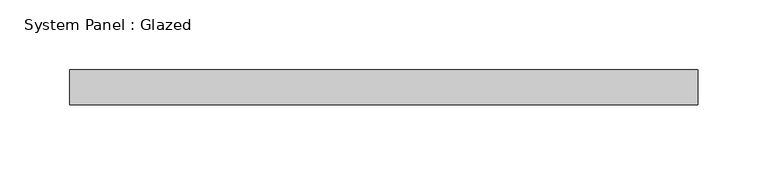
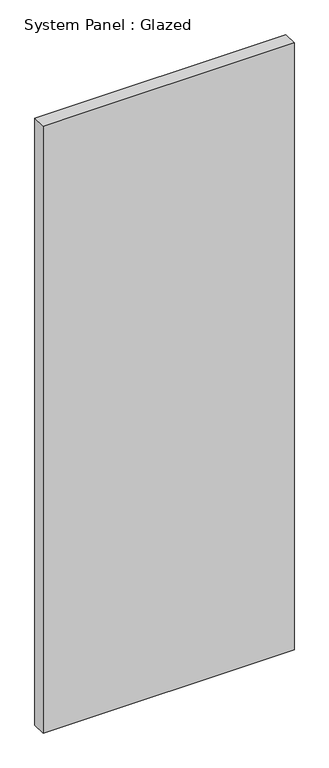
"""IFC4 building model written with IfcOpenShell, lengths in millimetres: plate geometry, System Panel : Glazed."""

from ifc_helpers import new_model, si_unit, origin, origin_with_axes, place, context, project, spatial, polyline, outline, extrude, source, transform, mapped, element, save


def system_panel_glazed_d4b66054(model_context):
    return source(origin(), model_context, "Body", "SweptSolid", [
        extrude(outline(polyline([(226.0465552, 19.05), (-226.0465552, 19.05), (-226.0465552, 44.45), (226.0465552, 44.45), (226.0465552, 19.05)])), origin_with_axes(), (0.0, 0.0, 1.0), 1155.7),
    ])


if __name__ == "__main__":
    model = new_model("IFC4")
    model_context = context("Model", 3, world=origin())
    ifc_project = project(units=[si_unit("LENGTHUNIT", "METRE", prefix="MILLI")], contexts=[model_context])
    site = spatial("IfcSite", under=ifc_project)
    building = spatial("IfcBuilding", under=site)
    placement = place(None, origin())
    system_panel_glazed_shape = system_panel_glazed_d4b66054(model_context)
    element("IfcPlate", 1, ObjectType="System Panel : Glazed", at=placement, inside=building, context=model_context, shape_type="MappedRepresentation", body=[
        mapped(system_panel_glazed_shape, transform((0.0, 0.0, 0.0), x_axis=(1.0, 0.0, 0.0), y_axis=(0.0, 1.0, 0.0), z_axis=(0.0, 0.0, 1.0))),
    ])
    save(model, "model.ifc")

# Revit data of these elements
# Type "System Panel : Glazed"
#   Construction Type Id = "GSP4R"
#   Analytic Construction = "1/8 in Pilkington single glazing"
#   Visual Light Transmittance = 0.9
#   Solar Heat Gain Coefficient = 0.86
#   Heat Transfer Coefficient (U) = 1.18115 BTU/(h·ft²·°F)
# Element 1 (IfcPlate, "System Panel : Glazed")
#   Materials on its faces: "Glass"
# Materials
#   "Glass": class "Glass", colour RGB 0 128 192, transparency 0.75, Description = "Soda Lime Glass", Cost = 0
